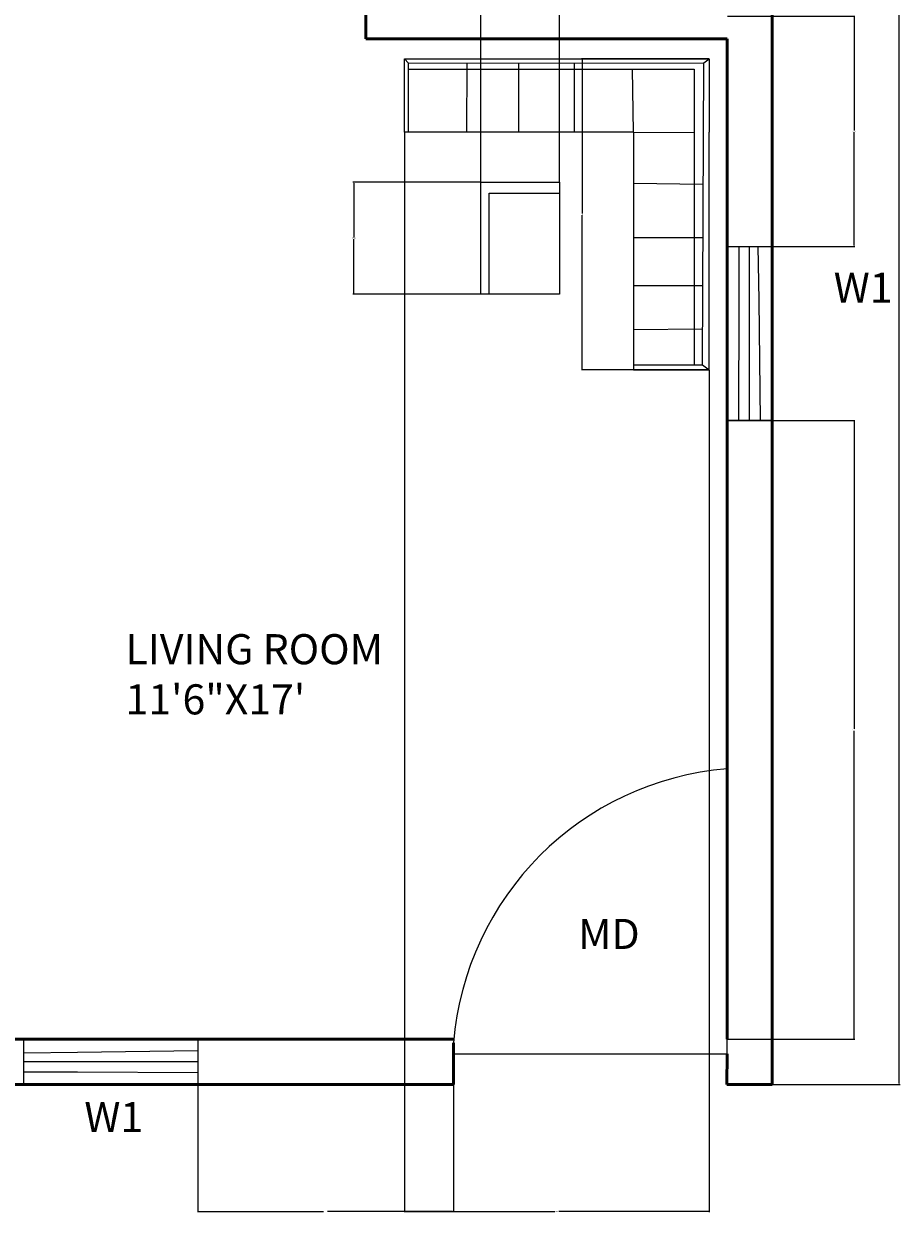
# Model space of a CAD drawing. Units: inches. Extents: x 2521 to 2933, y 1745 to 2276.
# Tile 2 of 4: x 2758 to 2933, y 1745 to 1982. Entities that reach past the tile are written whole.
import ezdxf

# ---------------------------------------------------------------- set-up
doc = ezdxf.new("R2010")
doc.units = ezdxf.units.IN
for name, color, linetype, lineweight in [('A-ANNO-DIMS', 2, 'Continuous', 18), ('A-ANNO-TEXT', 3, 'Continuous', 18), ('A-AREA-IDEN', 7, 'Continuous', 25), ('A-DOOR', 3, 'Continuous', 25), ('A-FURN', 8, 'Continuous', 18), ('A-GLAZ', 4, 'Continuous', 20), ('A-WALL', 7, 'Continuous', 50)]:
    doc.layers.add(name, color=color, linetype=linetype, lineweight=lineweight)
doc.styles.get("Standard").update_dxf_attribs({"font": 'arial.ttf'})
doc.dimstyles.get("Standard").update_dxf_attribs({"dimtxt": 0.18, "dimasz": 0.18, "dimexe": 0.18, "dimexo": 0.0625, "dimgap": 0.09, "dimtad": 0, "dimtih": 1, "dimtoh": 1, "dimdec": 4, "dimzin": 0, "dimdsep": 46, "dimtxsty": 'Standard', "dimcen": 0.09, "dimadec": 0, "dimazin": 0, "dimtfac": 1, "dimtdec": 4, "dimtofl": 0, "dimtmove": 0, "dimatfit": 3, "dimfxl": 1, "dimtolj": 1, "dimtzin": 0, "dimarcsym": 0})

# ---------------------------------------------------------------- blocks, each defined once
blk = doc.blocks.new('WINDOW-W1-LONG')
for p, q in [((0, 24), (0, 34.69)), ((0, 34.69), (9, 34.69)), ((2.4, 24), (2.44, 34.69)), ((4.5, 24), (4.5, 34.69)), ((6.37, 24), (6.23, 34.69)), ((9, 34.69), (9, 24)), ((0, 24), (0, 0)), ((2.32, 0), (2.4, 24)), ((4.5, 0), (4.5, 24)), ((6.68, 0), (6.37, 24)), ((9, 24), (9, 0)), ((9, 0), (0, 0))]:
    blk.add_line(p, q)
blk = doc.blocks.new('DOOR-SINGLE-SWING')
for p, q in [((54.54, 0), (54.54, 56.86)), ((0, 0), (54.54, 0))]:
    blk.add_line(p, q)
blk.add_arc((59.46, -2.59), 59.65, 94.7338, 175.398)
blk = doc.blocks.new('*D24')
at = {"layer": 'A-ANNO-DIMS', "color": 0, "lineweight": -2, "transparency": 16777216}
for p, q in [((2907.07, 2250.28), (2932.51, 2250.28)), ((2932.33, 2250.1), (2932.33, 2010.46)), ((2932.33, 1770.46), (2932.33, 2010.1)), ((2907.07, 1770.28), (2932.51, 1770.28))]:
    blk.add_line(p, q, dxfattribs=at)
at = {"layer": 'A-ANNO-DIMS', "color": 0, "transparency": 16777216}
for points in [[(2932.3, 2250.1), (2932.36, 2250.1), (2932.33, 2250.28)], [(2932.3, 1770.46), (2932.36, 1770.46), (2932.33, 1770.28)]]:
    blk.add_solid(points, dxfattribs=at)
at = {"layer": 'Defpoints', "color": 0, "transparency": 16777216}
for p in [(2907.01, 2250.28), (2932.33, 2250.28), (2907.01, 1770.28)]:
    blk.add_point(p, dxfattribs=at)
at = {"layer": 'A-ANNO-DIMS', "color": 0, "transparency": 16777216, "insert": (2932.33, 2010.28), "char_height": 0.18, "attachment_point": 5}
blk.add_mtext('\\A1;480', dxfattribs=at)
blk = doc.blocks.new('*D35')
at = {"layer": 'A-ANNO-DIMS', "color": 0, "lineweight": -2, "transparency": 16777216}
for p, q in [((2898.07, 1902.67), (2923.51, 1902.67)), ((2923.33, 1902.49), (2923.33, 1841.16)), ((2923.33, 1779.46), (2923.33, 1840.8)), ((2898.07, 1779.28), (2923.51, 1779.28))]:
    blk.add_line(p, q, dxfattribs=at)
at = {"layer": 'A-ANNO-DIMS', "color": 0, "transparency": 16777216}
for points in [[(2923.3, 1902.49), (2923.36, 1902.49), (2923.33, 1902.67)], [(2923.3, 1779.46), (2923.36, 1779.46), (2923.33, 1779.28)]]:
    blk.add_solid(points, dxfattribs=at)
at = {"layer": 'Defpoints', "color": 0, "transparency": 16777216}
for p in [(2898.01, 1902.67), (2898.01, 1779.28), (2923.33, 1779.28)]:
    blk.add_point(p, dxfattribs=at)
at = {"layer": 'A-ANNO-DIMS', "color": 0, "transparency": 16777216, "insert": (2923.33, 1840.98), "char_height": 0.18, "attachment_point": 5}
blk.add_mtext('\\A1;123.4', dxfattribs=at)
blk = doc.blocks.new('*D36')
at = {"layer": 'A-ANNO-DIMS', "color": 0, "lineweight": -2, "transparency": 16777216}
for p, q in [((2898.07, 1983.28), (2923.51, 1983.28)), ((2923.33, 1983.1), (2923.33, 1960.51)), ((2923.33, 1937.55), (2923.33, 1960.14)), ((2898.07, 1937.37), (2923.51, 1937.37))]:
    blk.add_line(p, q, dxfattribs=at)
at = {"layer": 'A-ANNO-DIMS', "color": 0, "transparency": 16777216}
for points in [[(2923.3, 1983.1), (2923.36, 1983.1), (2923.33, 1983.28)], [(2923.3, 1937.55), (2923.36, 1937.55), (2923.33, 1937.37)]]:
    blk.add_solid(points, dxfattribs=at)
at = {"layer": 'Defpoints', "color": 0, "transparency": 16777216}
for p in [(2898.01, 1983.28), (2898.01, 1937.37), (2923.33, 1937.37)]:
    blk.add_point(p, dxfattribs=at)
at = {"layer": 'A-ANNO-DIMS', "color": 0, "transparency": 16777216, "insert": (2923.33, 1960.32), "char_height": 0.18, "attachment_point": 5}
blk.add_mtext('\\A1;45.91', dxfattribs=at)
blk = doc.blocks.new('*D44')
at = {"layer": 'A-ANNO-DIMS', "color": 0, "lineweight": -2, "transparency": 16777216}
for p, q in [((2792.49, 1770.22), (2792.49, 1744.78)), ((2843.47, 1770.22), (2843.47, 1744.78)), ((2792.67, 1744.96), (2817.58, 1744.96)), ((2843.29, 1744.96), (2818.37, 1744.96))]:
    blk.add_line(p, q, dxfattribs=at)
at = {"layer": 'A-ANNO-DIMS', "color": 0, "transparency": 16777216}
for points in [[(2792.67, 1744.99), (2792.67, 1744.93), (2792.49, 1744.96)], [(2843.29, 1744.99), (2843.29, 1744.93), (2843.47, 1744.96)]]:
    blk.add_solid(points, dxfattribs=at)
at = {"layer": 'Defpoints', "color": 0, "transparency": 16777216}
for p in [(2792.49, 1770.28), (2843.47, 1770.28), (2843.47, 1744.96)]:
    blk.add_point(p, dxfattribs=at)
at = {"layer": 'A-ANNO-DIMS', "color": 0, "transparency": 16777216, "insert": (2817.98, 1744.96), "char_height": 0.18, "attachment_point": 5}
blk.add_mtext('\\A1;50.98', dxfattribs=at)
blk = doc.blocks.new('*D57')
at = {"layer": 'A-ANNO-DIMS', "color": 0, "lineweight": -2, "transparency": 16777216}
for p, q in [((2833.68, 1960.07), (2833.68, 1744.78)), ((2894.46, 1912.71), (2894.46, 1744.78)), ((2833.86, 1744.96), (2863.68, 1744.96)), ((2894.28, 1744.96), (2864.47, 1744.96))]:
    blk.add_line(p, q, dxfattribs=at)
at = {"layer": 'A-ANNO-DIMS', "color": 0, "transparency": 16777216}
for points in [[(2833.86, 1744.99), (2833.86, 1744.93), (2833.68, 1744.96)], [(2894.28, 1744.99), (2894.28, 1744.93), (2894.46, 1744.96)]]:
    blk.add_solid(points, dxfattribs=at)
at = {"layer": 'Defpoints', "color": 0, "transparency": 16777216}
for p in [(2833.68, 1960.13), (2894.46, 1912.77), (2894.46, 1744.96)]:
    blk.add_point(p, dxfattribs=at)
at = {"layer": 'A-ANNO-DIMS', "color": 0, "transparency": 16777216, "insert": (2864.07, 1744.96), "char_height": 0.18, "attachment_point": 5}
blk.add_mtext('\\A1;60.78', dxfattribs=at)
blk = doc.blocks.new('*D58')
at = {"layer": 'A-ANNO-DIMS', "color": 0, "lineweight": -2, "transparency": 16777216}
for p, q in [((2894.4, 1974.77), (2868.96, 1974.77)), ((2869.14, 1974.59), (2869.14, 1943.96)), ((2869.14, 1912.95), (2869.14, 1943.59)), ((2894.4, 1912.77), (2868.96, 1912.77))]:
    blk.add_line(p, q, dxfattribs=at)
at = {"layer": 'A-ANNO-DIMS', "color": 0, "transparency": 16777216}
for points in [[(2869.11, 1974.59), (2869.17, 1974.59), (2869.14, 1974.77)], [(2869.11, 1912.95), (2869.17, 1912.95), (2869.14, 1912.77)]]:
    blk.add_solid(points, dxfattribs=at)
at = {"layer": 'Defpoints', "color": 0, "transparency": 16777216}
for p in [(2869.14, 1974.77), (2894.46, 1974.77), (2894.46, 1912.77)]:
    blk.add_point(p, dxfattribs=at)
at = {"layer": 'A-ANNO-DIMS', "color": 0, "transparency": 16777216, "insert": (2869.14, 1943.77), "char_height": 0.18, "attachment_point": 5}
blk.add_mtext('\\A1;62', dxfattribs=at)
blk = doc.blocks.new('*D59')
at = {"layer": 'A-ANNO-DIMS', "color": 0, "lineweight": -2, "transparency": 16777216}
for p, q in [((2848.92, 1927.91), (2848.92, 2275.78)), ((2849.1, 2275.6), (2856.29, 2275.6)), ((2864.39, 2275.6), (2857.2, 2275.6)), ((2864.57, 1950.23), (2864.57, 2275.78))]:
    blk.add_line(p, q, dxfattribs=at)
at = {"layer": 'A-ANNO-DIMS', "color": 0, "transparency": 16777216}
for points in [[(2849.1, 2275.63), (2849.1, 2275.57), (2848.92, 2275.6)], [(2864.39, 2275.63), (2864.39, 2275.57), (2864.57, 2275.6)]]:
    blk.add_solid(points, dxfattribs=at)
at = {"layer": 'Defpoints', "color": 0, "transparency": 16777216}
for p in [(2864.57, 2275.6), (2864.57, 1950.17), (2848.92, 1927.85)]:
    blk.add_point(p, dxfattribs=at)
at = {"layer": 'A-ANNO-DIMS', "color": 0, "transparency": 16777216, "insert": (2856.74, 2275.6), "char_height": 0.18, "attachment_point": 5}
blk.add_mtext('\\A1;15.656', dxfattribs=at)
blk = doc.blocks.new('*D60')
at = {"layer": 'A-ANNO-DIMS', "color": 0, "lineweight": -2, "transparency": 16777216}
for p, q in [((2848.85, 1950.17), (2823.42, 1950.17)), ((2823.6, 1949.99), (2823.6, 1939.19)), ((2823.6, 1928.03), (2823.6, 1938.83)), ((2848.85, 1927.85), (2823.42, 1927.85))]:
    blk.add_line(p, q, dxfattribs=at)
at = {"layer": 'A-ANNO-DIMS', "color": 0, "transparency": 16777216}
for points in [[(2823.57, 1949.99), (2823.63, 1949.99), (2823.6, 1950.17)], [(2823.57, 1928.03), (2823.63, 1928.03), (2823.6, 1927.85)]]:
    blk.add_solid(points, dxfattribs=at)
at = {"layer": 'Defpoints', "color": 0, "transparency": 16777216}
for p in [(2823.6, 1950.17), (2848.92, 1950.17), (2848.92, 1927.85)]:
    blk.add_point(p, dxfattribs=at)
at = {"layer": 'A-ANNO-DIMS', "color": 0, "transparency": 16777216, "insert": (2823.6, 1939.01), "char_height": 0.18, "attachment_point": 5}
blk.add_mtext('\\A1;22.325', dxfattribs=at)

msp = doc.modelspace()

# ---------------------------------------------------------------- linework, layer by layer
at = {"layer": 'A-FURN'}
for p, q in [((2833.6831, 1974.7747), (2834.508, 1973.9428)), ((2893.3494, 1974.0224), (2894.4636, 1974.7747)), ((2834.4854, 1960.1324), (2834.508, 1973.9428)), ((2834.506, 1972.7285), (2891.4329, 1972.7285)), ((2834.508, 1973.9428), (2893.3494, 1974.0224)), ((2846.1603, 1960.1324), (2846.1782, 1973.9586)), ((2856.5059, 1960.1324), (2856.4713, 1973.9725)), ((2867.5603, 1960.1324), (2867.56, 1973.9875)), ((2879.3288, 1960.1324), (2879.163, 1972.7285)), ((2891.4329, 1972.7285), (2891.4329, 1913.8009)), ((2893.0902, 1913.8009), (2893.3494, 1974.0224)), ((2879.3288, 1960.1324), (2891.4329, 1960.0828)), ((2879.3288, 1949.9669), (2893.2452, 1949.8173)), ((2850.5749, 1927.8472), (2850.5749, 1947.9992)), ((2850.5749, 1947.9992), (2851.5792, 1947.9992)), ((2851.5792, 1947.9992), (2864.5724, 1947.9992)), ((2879.3288, 1939.1832), (2893.1994, 1939.1828)), ((2879.3288, 1929.5885), (2893.1582, 1929.6046)), ((2879.3288, 1920.8279), (2893.1211, 1920.9766)), ((2879.3288, 1913.8009), (2893.0902, 1913.8009)), ((2893.0902, 1913.8009), (2894.4636, 1912.7746))]:
    msp.add_line(p, q, dxfattribs=at)
for points in [[(2879.3288, 1960.1324), (2833.6831, 1960.1324), (2833.6831, 1974.7747), (2894.4636, 1974.7747), (2894.4636, 1960.1324)], [(2879.3288, 1960.1324), (2879.3288, 1912.7746), (2894.4636, 1912.7746), (2894.4636, 1960.1324)]]:
    msp.add_lwpolyline(points, dxfattribs=at)
msp.add_lwpolyline([(2848.9165, 1950.1723), (2864.5724, 1950.1723), (2864.5724, 1927.8472), (2848.9165, 1927.8472)], close=True, dxfattribs=at)
at = {"layer": 'A-WALL'}
for p, q in [((2907.009, 2250.2819), (2907.009, 1770.2819)), ((2826.009, 1980.2819), (2826.009, 2076.2819)), ((2826.009, 1980.2819), (2826.009, 1978.7819)), ((2826.009, 1978.7819), (2898.009, 1978.7819)), ((2898.009, 1978.7819), (2898.009, 1779.2819)), ((2843.3859, 1779.2819), (2739.009, 1779.2819)), ((2843.3859, 1779.2819), (2760.009, 1779.2819)), ((2843.4735, 1778.5611), (2843.4735, 1776.3642)), ((2843.4735, 1776.3642), (2843.4686, 1770.2819)), ((2898.009, 1776.3642), (2897.9721, 1770.2819)), ((2843.4686, 1770.2819), (2547.009, 1770.2819)), ((2843.4686, 1770.2819), (2769.009, 1770.2819)), ((2907.009, 1770.2819), (2897.9721, 1770.2819)), ((2907.009, 1770.2819), (2897.9721, 1770.2819))]:
    msp.add_line(p, q, dxfattribs=at)

# ---------------------------------------------------------------- block references
at = {"layer": 'A-DOOR'}
msp.add_blockref('DOOR-SINGLE-SWING', (2843.473, 1776.3642), dxfattribs=at)
at = {"layer": 'A-GLAZ'}
msp.add_blockref('WINDOW-W1-LONG', (2898.009, 1902.6733), dxfattribs=at)
at = {"layer": 'A-GLAZ', "rotation": 90}
msp.add_blockref('WINDOW-W1-LONG', (2792.4883, 1770.2819), dxfattribs=at)

# ---------------------------------------------------------------- texts
at = {"layer": 'A-ANNO-TEXT', "char_height": 6, "attachment_point": 1}
for s, width, insert in [('W1', 12.996108, (2919.2739, 1932.1429)), ('MD', 13.154301, (2868.3124, 1803.2764)), ('W1', 10.875604, (2769.8735, 1766.7576))]:
    msp.add_mtext_dynamic_manual_height_columns(s, width=width, gutter_width=5.8967, heights=[0], dxfattribs=dict(at, insert=insert))
at = {"layer": 'A-AREA-IDEN', "insert": (2778.0789, 1860.0605), "char_height": 6, "attachment_point": 1}
msp.add_mtext_dynamic_manual_height_columns('LIVING ROOM \\P11\'6"X17\'', width=69.183519, gutter_width=5.8967, heights=[0], dxfattribs=at)

# ---------------------------------------------------------------- dimensions: what is measured, and where the dimension line sits
at = {"layer": 'A-ANNO-DIMS'}
for base, p1, p2, override, picture, middle in [((2864.5724, 2275.6019), (2848.9165, 1927.8472), (2864.5724, 1950.1723), {"dimdec": 3, "dimlfac": 1, "dimrnd": 0, "dimzin": 0, "dimdsep": 46, "dimlunit": 2}, '*D59', (2856.7445, 2275.6019)), ((2894.4636, 1744.9619), (2833.6831, 1960.1324), (2894.4636, 1912.7746), {"dimdec": 2, "dimlfac": 1, "dimrnd": 0, "dimzin": 0, "dimdsep": 46, "dimlunit": 2}, '*D57', (2864.0734, 1744.9619)), ((2843.4686, 1744.9619), (2792.4881, 1770.2819), (2843.4686, 1770.2819), {"dimdec": 2, "dimlfac": 1, "dimrnd": 0, "dimzin": 0, "dimdsep": 46, "dimlunit": 2}, '*D44', (2817.9784, 1744.9619))]:
    dim = msp.add_linear_dim(base=base, p1=p1, p2=p2, dimstyle='Standard', override=override, dxfattribs=at)
    dim.commit()
    dim.dimension.update_dxf_attribs({"geometry": picture, "text_midpoint": middle})
for base, p1, p2, angle, override, picture, middle in [((2932.329, 2250.2819), (2907.009, 1770.2819), (2907.009, 2250.2819), 90, {"dimdec": 0, "dimlfac": 1, "dimrnd": 0, "dimzin": 0, "dimdsep": 46, "dimlunit": 2}, '*D24', (2932.329, 2010.2819)), ((2923.329, 1937.3677), (2898.009, 1983.2819), (2898.009, 1937.3677), 270, {"dimdec": 2, "dimlfac": 1, "dimrnd": 0, "dimzin": 0, "dimdsep": 46, "dimlunit": 2}, '*D36', (2923.329, 1960.3248)), ((2869.1436, 1974.7747), (2894.4636, 1912.7746), (2894.4636, 1974.7747), 90, {"dimdec": 0, "dimlfac": 1, "dimrnd": 0, "dimzin": 0, "dimdsep": 46, "dimlunit": 2}, '*D58', (2869.1436, 1943.7747)), ((2823.5965, 1950.1723), (2848.9165, 1927.8472), (2848.9165, 1950.1723), 90, {"dimdec": 3, "dimlfac": 1, "dimrnd": 0, "dimzin": 0, "dimdsep": 46, "dimlunit": 2}, '*D60', (2823.5965, 1939.0098)), ((2923.329, 1779.2819), (2898.009, 1902.6735), (2898.009, 1779.2819), 270, {"dimdec": 1, "dimlfac": 1, "dimrnd": 0, "dimzin": 0, "dimdsep": 46, "dimlunit": 2}, '*D35', (2923.329, 1840.9777))]:
    dim = msp.add_linear_dim(base=base, p1=p1, p2=p2, angle=angle, dimstyle='Standard', override=override, dxfattribs=at)
    dim.commit()
    dim.dimension.update_dxf_attribs({"geometry": picture, "text_midpoint": middle})

doc.saveas('drawing.dxf')
